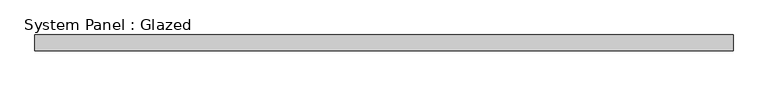
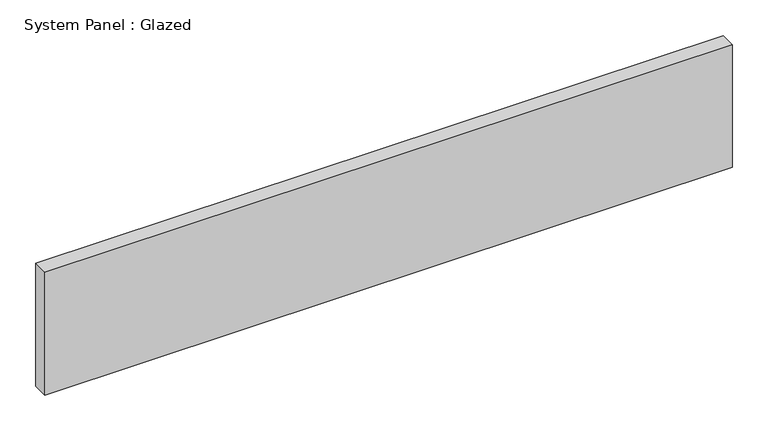
"""IFC4 building model written with IfcOpenShell, lengths in millimetres: plate geometry, System Panel : Glazed."""

from ifc_helpers import new_model, si_unit, origin, origin_with_axes, place, context, project, spatial, polyline, outline, extrude, source, transform, mapped, element, save


def system_panel_glazed_d7074436(model_context):
    return source(origin(), model_context, "Body", "SweptSolid", [
        extrude(outline(polyline([(555.625, 19.05), (-555.625, 19.05), (-555.625, 44.45), (555.625, 44.45), (555.625, 19.05)])), origin_with_axes(), (0.0, 0.0, 1.0), 209.55),
    ])


if __name__ == "__main__":
    model = new_model("IFC4")
    model_context = context("Model", 3, world=origin())
    ifc_project = project(units=[si_unit("LENGTHUNIT", "METRE", prefix="MILLI")], contexts=[model_context])
    site = spatial("IfcSite", under=ifc_project)
    building = spatial("IfcBuilding", under=site)
    placement = place(None, origin())
    system_panel_glazed_shape = system_panel_glazed_d7074436(model_context)
    element("IfcPlate", 1, ObjectType="System Panel : Glazed", at=placement, inside=building, context=model_context, shape_type="MappedRepresentation", body=[
        mapped(system_panel_glazed_shape, transform((0.0, 0.0, 0.0), x_axis=(1.0, 0.0, 0.0), y_axis=(0.0, 1.0, 0.0), z_axis=(0.0, 0.0, 1.0))),
    ])
    save(model, "model.ifc")

# Revit data of these elements
# Type "System Panel : Glazed"
#   Construction Type Id = "GSP4R"
#   Analytic Construction = "1/8 in Pilkington single glazing"
#   Visual Light Transmittance = 0.9
#   Solar Heat Gain Coefficient = 0.86
#   Heat Transfer Coefficient (U) = 1.18115 BTU/(h·ft²·°F)
#   Define Thermal Properties by = 1
# Element 1 (IfcPlate, "System Panel : Glazed")
#   Materials on its faces: "Glass"
# Materials
#   "Glass": class "Glass", colour RGB 0 128 192, transparency 0.75, Description = "Soda Lime Glass", Cost = 0
